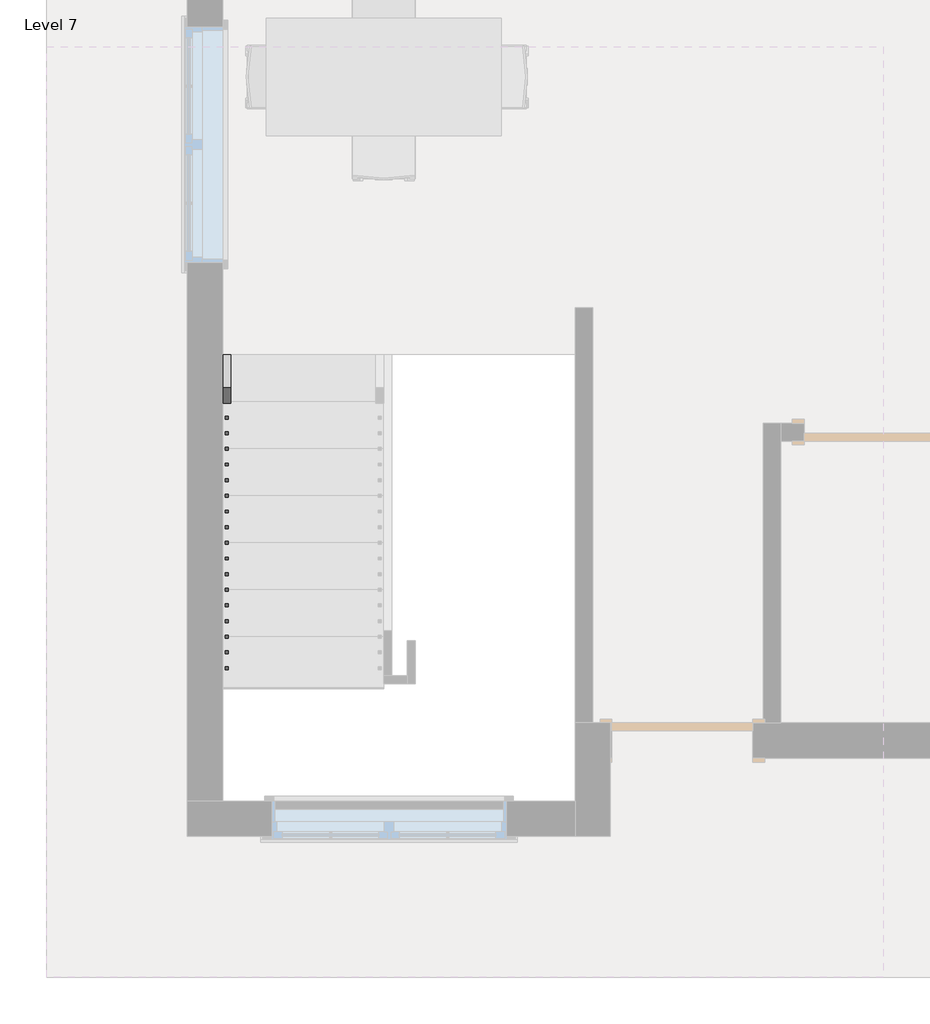
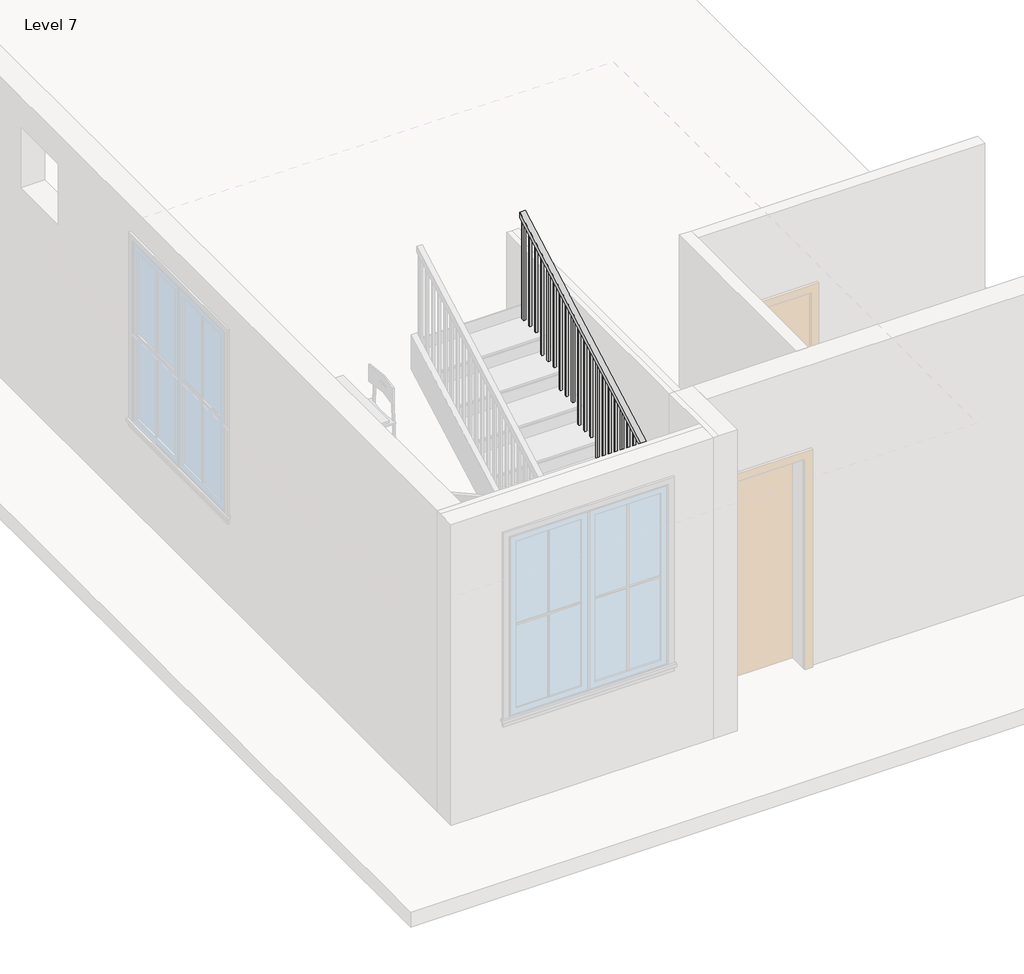
# One storey, part 2 of 3: 1 railing.
"""IFC4 building model written with IfcOpenShell, lengths in millimetres."""

from ifc_helpers import new_model, si_unit, frame, origin, place, context, project, spatial, polyline, outline, extrude, faceted_brep, element, save

model = new_model("IFC4")

# Units and contexts
model_context = context("Model", 3, world=origin())
ifc_project = project(units=[si_unit("LENGTHUNIT", "METRE", prefix="MILLI")], contexts=[model_context])

# Site, building, storey
site = spatial("IfcSite", under=ifc_project)
building = spatial("IfcBuilding", under=site)
storey = spatial("IfcBuildingStorey", under=building, Name="Level 7", Elevation=19050.0)

# Railing
placement = place(None, origin())
element("IfcRailing", 1, ObjectType="Handrail - Rectangular", at=placement, inside=storey, context=model_context, shape_type="SolidModel", body=[
    faceted_brep([(-4181.480864, -3571.6080018, 20133.7333333), (-4181.480864, -3571.6080018, 20075.620221), (-4232.280864, -3571.6080018, 20075.620221), (-4232.280864, -3571.6080018, 20133.7333333), (-4181.480864, -5705.2080018, 21319.0666667), (-4181.480864, -5718.371604, 21268.2666667), (-4232.280864, -5718.371604, 21268.2666667), (-4232.280864, -5705.2080018, 21319.0666667), (-4181.480864, -6416.4080018, 21319.0666667), (-4181.480864, -6416.4080018, 21268.2666667), (-4232.280864, -6467.2080018, 21268.2666667), (-4232.280864, -6467.2080018, 21319.0666667), (-1997.080864, -6416.4080018, 21319.0666667), (-1997.080864, -6416.4080018, 21268.2666667), (-1946.280864, -6467.2080018, 21268.2666667), (-1946.280864, -6467.2080018, 21319.0666667), (-1997.080864, -5705.2080018, 21319.0666667), (-1997.080864, -5692.0443995, 21268.2666667), (-1946.280864, -5692.0443995, 21268.2666667), (-1946.280864, -5705.2080018, 21319.0666667), (-1997.080864, -3571.6080018, 22504.4), (-1946.280864, -3571.6080018, 22504.4), (-1946.280864, -3571.6080018, 22446.2868876), (-1997.080864, -3571.6080018, 22446.2868876)], [[[0, 1, 2, 3]], [[1, 0, 4, 5]], [[2, 1, 5, 6]], [[3, 2, 6, 7]], [[0, 3, 7, 4]], [[5, 4, 8, 9]], [[6, 5, 9, 10]], [[7, 6, 10, 11]], [[4, 7, 11, 8]], [[9, 8, 12, 13]], [[10, 9, 13, 14]], [[11, 10, 14, 15]], [[8, 11, 15, 12]], [[13, 12, 16, 17]], [[14, 13, 17, 18]], [[15, 14, 18, 19]], [[12, 15, 19, 16]], [[20, 21, 22, 23]], [[17, 16, 20, 23]], [[18, 17, 23, 22]], [[19, 18, 22, 21]], [[16, 19, 21, 20]]]),
    extrude(outline(polyline([(-3606.5330018, 22426.8841099), (-3587.4830018, 22437.4674432), (-3587.4830018, 21420.6666667), (-3606.5330018, 21420.6666667), (-3606.5330018, 22426.8841099)])), frame((-1981.205864, 0.0, 0.0), z_axis=(1.0, 0.0, 0.0), x_axis=(0.0, 1.0, 0.0)), (0.0, 0.0, 1.0), 19.05),
    extrude(outline(polyline([(-3708.1330018, 22370.4396654), (-3689.0830018, 22381.0229988), (-3689.0830018, 21420.6666667), (-3708.1330018, 21420.6666667), (-3708.1330018, 22370.4396654)])), frame((-1981.205864, 0.0, 0.0), z_axis=(1.0, 0.0, 0.0), x_axis=(0.0, 1.0, 0.0)), (0.0, 0.0, 1.0), 19.05),
    extrude(outline(polyline([(-3809.7330018, 22313.995221), (-3790.6830018, 22324.5785543), (-3790.6830018, 21420.6666667), (-3809.7330018, 21420.6666667), (-3809.7330018, 22313.995221)])), frame((-1981.205864, 0.0, 0.0), z_axis=(1.0, 0.0, 0.0), x_axis=(0.0, 1.0, 0.0)), (0.0, 0.0, 1.0), 19.05),
    extrude(outline(polyline([(-3911.3330018, 22257.5507765), (-3892.2830018, 22268.1341099), (-3892.2830018, 21251.3333333), (-3911.3330018, 21251.3333333), (-3911.3330018, 22257.5507765)])), frame((-1981.205864, 0.0, 0.0), z_axis=(1.0, 0.0, 0.0), x_axis=(0.0, 1.0, 0.0)), (0.0, 0.0, 1.0), 19.05),
    extrude(outline(polyline([(-4012.9330018, 22201.1063321), (-3993.8830018, 22211.6896654), (-3993.8830018, 21251.3333333), (-4012.9330018, 21251.3333333), (-4012.9330018, 22201.1063321)])), frame((-1981.205864, 0.0, 0.0), z_axis=(1.0, 0.0, 0.0), x_axis=(0.0, 1.0, 0.0)), (0.0, 0.0, 1.0), 19.05),
    extrude(outline(polyline([(-4114.5330018, 22144.6618876), (-4095.4830018, 22155.245221), (-4095.4830018, 21251.3333333), (-4114.5330018, 21251.3333333), (-4114.5330018, 22144.6618876)])), frame((-1981.205864, 0.0, 0.0), z_axis=(1.0, 0.0, 0.0), x_axis=(0.0, 1.0, 0.0)), (0.0, 0.0, 1.0), 19.05),
    extrude(outline(polyline([(-4216.1330018, 22088.2174432), (-4197.0830018, 22098.8007765), (-4197.0830018, 21082.0), (-4216.1330018, 21082.0), (-4216.1330018, 22088.2174432)])), frame((-1981.205864, 0.0, 0.0), z_axis=(1.0, 0.0, 0.0), x_axis=(0.0, 1.0, 0.0)), (0.0, 0.0, 1.0), 19.05),
    extrude(outline(polyline([(-4317.7330018, 22031.7729988), (-4298.6830018, 22042.3563321), (-4298.6830018, 21082.0), (-4317.7330018, 21082.0), (-4317.7330018, 22031.7729988)])), frame((-1981.205864, 0.0, 0.0), z_axis=(1.0, 0.0, 0.0), x_axis=(0.0, 1.0, 0.0)), (0.0, 0.0, 1.0), 19.05),
    extrude(outline(polyline([(-4419.3330018, 21975.3285543), (-4400.2830018, 21985.9118876), (-4400.2830018, 21082.0), (-4419.3330018, 21082.0), (-4419.3330018, 21975.3285543)])), frame((-1981.205864, 0.0, 0.0), z_axis=(1.0, 0.0, 0.0), x_axis=(0.0, 1.0, 0.0)), (0.0, 0.0, 1.0), 19.05),
    extrude(outline(polyline([(-4520.9330018, 21918.8841099), (-4501.8830018, 21929.4674432), (-4501.8830018, 20912.6666667), (-4520.9330018, 20912.6666667), (-4520.9330018, 21918.8841099)])), frame((-1981.205864, 0.0, 0.0), z_axis=(1.0, 0.0, 0.0), x_axis=(0.0, 1.0, 0.0)), (0.0, 0.0, 1.0), 19.05),
    extrude(outline(polyline([(-4622.5330018, 21862.4396654), (-4603.4830018, 21873.0229988), (-4603.4830018, 20912.6666667), (-4622.5330018, 20912.6666667), (-4622.5330018, 21862.4396654)])), frame((-1981.205864, 0.0, 0.0), z_axis=(1.0, 0.0, 0.0), x_axis=(0.0, 1.0, 0.0)), (0.0, 0.0, 1.0), 19.05),
    extrude(outline(polyline([(-4724.1330018, 21805.995221), (-4705.0830018, 21816.5785543), (-4705.0830018, 20912.6666667), (-4724.1330018, 20912.6666667), (-4724.1330018, 21805.995221)])), frame((-1981.205864, 0.0, 0.0), z_axis=(1.0, 0.0, 0.0), x_axis=(0.0, 1.0, 0.0)), (0.0, 0.0, 1.0), 19.05),
    extrude(outline(polyline([(-4825.7330018, 21749.5507765), (-4806.6830018, 21760.1341099), (-4806.6830018, 20743.3333333), (-4825.7330018, 20743.3333333), (-4825.7330018, 21749.5507765)])), frame((-1981.205864, 0.0, 0.0), z_axis=(1.0, 0.0, 0.0), x_axis=(0.0, 1.0, 0.0)), (0.0, 0.0, 1.0), 19.05),
    extrude(outline(polyline([(-4927.3330018, 21693.1063321), (-4908.2830018, 21703.6896654), (-4908.2830018, 20743.3333333), (-4927.3330018, 20743.3333333), (-4927.3330018, 21693.1063321)])), frame((-1981.205864, 0.0, 0.0), z_axis=(1.0, 0.0, 0.0), x_axis=(0.0, 1.0, 0.0)), (0.0, 0.0, 1.0), 19.05),
    extrude(outline(polyline([(-5028.9330018, 21636.6618876), (-5009.8830018, 21647.245221), (-5009.8830018, 20743.3333333), (-5028.9330018, 20743.3333333), (-5028.9330018, 21636.6618876)])), frame((-1981.205864, 0.0, 0.0), z_axis=(1.0, 0.0, 0.0), x_axis=(0.0, 1.0, 0.0)), (0.0, 0.0, 1.0), 19.05),
    extrude(outline(polyline([(-5130.5330018, 21580.2174432), (-5111.4830018, 21590.8007765), (-5111.4830018, 20574.0), (-5130.5330018, 20574.0), (-5130.5330018, 21580.2174432)])), frame((-1981.205864, 0.0, 0.0), z_axis=(1.0, 0.0, 0.0), x_axis=(0.0, 1.0, 0.0)), (0.0, 0.0, 1.0), 19.05),
    extrude(outline(polyline([(-5232.1330018, 21523.7729988), (-5213.0830018, 21534.3563321), (-5213.0830018, 20574.0), (-5232.1330018, 20574.0), (-5232.1330018, 21523.7729988)])), frame((-1981.205864, 0.0, 0.0), z_axis=(1.0, 0.0, 0.0), x_axis=(0.0, 1.0, 0.0)), (0.0, 0.0, 1.0), 19.05),
    extrude(outline(polyline([(-5333.7330018, 21467.3285543), (-5314.6830018, 21477.9118876), (-5314.6830018, 20574.0), (-5333.7330018, 20574.0), (-5333.7330018, 21467.3285543)])), frame((-1981.205864, 0.0, 0.0), z_axis=(1.0, 0.0, 0.0), x_axis=(0.0, 1.0, 0.0)), (0.0, 0.0, 1.0), 19.05),
    extrude(outline(polyline([(-5435.3330018, 21410.8841099), (-5416.2830018, 21421.4674432), (-5416.2830018, 20404.6666667), (-5435.3330018, 20404.6666667), (-5435.3330018, 21410.8841099)])), frame((-1981.205864, 0.0, 0.0), z_axis=(1.0, 0.0, 0.0), x_axis=(0.0, 1.0, 0.0)), (0.0, 0.0, 1.0), 19.05),
    extrude(outline(polyline([(-5536.9330018, 21354.4396654), (-5517.8830018, 21365.0229988), (-5517.8830018, 20404.6666667), (-5536.9330018, 20404.6666667), (-5536.9330018, 21354.4396654)])), frame((-1981.205864, 0.0, 0.0), z_axis=(1.0, 0.0, 0.0), x_axis=(0.0, 1.0, 0.0)), (0.0, 0.0, 1.0), 19.05),
    extrude(outline(polyline([(-5638.5330018, 21297.995221), (-5619.4830018, 21308.5785543), (-5619.4830018, 20404.6666667), (-5638.5330018, 20404.6666667), (-5638.5330018, 21297.995221)])), frame((-1981.205864, 0.0, 0.0), z_axis=(1.0, 0.0, 0.0), x_axis=(0.0, 1.0, 0.0)), (0.0, 0.0, 1.0), 19.05),
    extrude(outline(polyline([(-1962.155864, -5740.1330018), (-1981.205864, -5740.1330018), (-1981.205864, -5721.0830018), (-1962.155864, -5721.0830018), (-1962.155864, -5740.1330018)])), frame((0.0, 0.0, 20404.6666667), z_axis=(0.0, 0.0, 1.0), x_axis=(1.0, 0.0, 0.0)), (0.0, 0.0, 1.0), 863.6),
    extrude(outline(polyline([(-1962.155864, -5841.7330018), (-1981.205864, -5841.7330018), (-1981.205864, -5822.6830018), (-1962.155864, -5822.6830018), (-1962.155864, -5841.7330018)])), frame((0.0, 0.0, 20404.6666667), z_axis=(0.0, 0.0, 1.0), x_axis=(1.0, 0.0, 0.0)), (0.0, 0.0, 1.0), 863.6),
    extrude(outline(polyline([(-1962.155864, -5943.3330018), (-1981.205864, -5943.3330018), (-1981.205864, -5924.2830018), (-1962.155864, -5924.2830018), (-1962.155864, -5943.3330018)])), frame((0.0, 0.0, 20404.6666667), z_axis=(0.0, 0.0, 1.0), x_axis=(1.0, 0.0, 0.0)), (0.0, 0.0, 1.0), 863.6),
    extrude(outline(polyline([(-1962.155864, -6044.9330018), (-1981.205864, -6044.9330018), (-1981.205864, -6025.8830018), (-1962.155864, -6025.8830018), (-1962.155864, -6044.9330018)])), frame((0.0, 0.0, 20404.6666667), z_axis=(0.0, 0.0, 1.0), x_axis=(1.0, 0.0, 0.0)), (0.0, 0.0, 1.0), 863.6),
    extrude(outline(polyline([(-1962.155864, -6146.5330018), (-1981.205864, -6146.5330018), (-1981.205864, -6127.4830018), (-1962.155864, -6127.4830018), (-1962.155864, -6146.5330018)])), frame((0.0, 0.0, 20404.6666667), z_axis=(0.0, 0.0, 1.0), x_axis=(1.0, 0.0, 0.0)), (0.0, 0.0, 1.0), 863.6),
    extrude(outline(polyline([(-1962.155864, -6248.1330018), (-1981.205864, -6248.1330018), (-1981.205864, -6229.0830018), (-1962.155864, -6229.0830018), (-1962.155864, -6248.1330018)])), frame((0.0, 0.0, 20404.6666667), z_axis=(0.0, 0.0, 1.0), x_axis=(1.0, 0.0, 0.0)), (0.0, 0.0, 1.0), 863.6),
    extrude(outline(polyline([(-1962.155864, -6349.7330018), (-1981.205864, -6349.7330018), (-1981.205864, -6330.6830018), (-1962.155864, -6330.6830018), (-1962.155864, -6349.7330018)])), frame((0.0, 0.0, 20404.6666667), z_axis=(0.0, 0.0, 1.0), x_axis=(1.0, 0.0, 0.0)), (0.0, 0.0, 1.0), 863.6),
    extrude(outline(polyline([(-2082.805864, -6451.3330018), (-2082.805864, -6432.2830018), (-2063.755864, -6432.2830018), (-2063.755864, -6451.3330018), (-2082.805864, -6451.3330018)])), frame((0.0, 0.0, 20404.6666667), z_axis=(0.0, 0.0, 1.0), x_axis=(1.0, 0.0, 0.0)), (0.0, 0.0, 1.0), 863.6),
    extrude(outline(polyline([(-2184.405864, -6451.3330018), (-2184.405864, -6432.2830018), (-2165.355864, -6432.2830018), (-2165.355864, -6451.3330018), (-2184.405864, -6451.3330018)])), frame((0.0, 0.0, 20404.6666667), z_axis=(0.0, 0.0, 1.0), x_axis=(1.0, 0.0, 0.0)), (0.0, 0.0, 1.0), 863.6),
    extrude(outline(polyline([(-2286.005864, -6451.3330018), (-2286.005864, -6432.2830018), (-2266.955864, -6432.2830018), (-2266.955864, -6451.3330018), (-2286.005864, -6451.3330018)])), frame((0.0, 0.0, 20404.6666667), z_axis=(0.0, 0.0, 1.0), x_axis=(1.0, 0.0, 0.0)), (0.0, 0.0, 1.0), 863.6),
    extrude(outline(polyline([(-2387.605864, -6451.3330018), (-2387.605864, -6432.2830018), (-2368.555864, -6432.2830018), (-2368.555864, -6451.3330018), (-2387.605864, -6451.3330018)])), frame((0.0, 0.0, 20404.6666667), z_axis=(0.0, 0.0, 1.0), x_axis=(1.0, 0.0, 0.0)), (0.0, 0.0, 1.0), 863.6),
    extrude(outline(polyline([(-2489.205864, -6451.3330018), (-2489.205864, -6432.2830018), (-2470.155864, -6432.2830018), (-2470.155864, -6451.3330018), (-2489.205864, -6451.3330018)])), frame((0.0, 0.0, 20404.6666667), z_axis=(0.0, 0.0, 1.0), x_axis=(1.0, 0.0, 0.0)), (0.0, 0.0, 1.0), 863.6),
    extrude(outline(polyline([(-2590.805864, -6451.3330018), (-2590.805864, -6432.2830018), (-2571.755864, -6432.2830018), (-2571.755864, -6451.3330018), (-2590.805864, -6451.3330018)])), frame((0.0, 0.0, 20404.6666667), z_axis=(0.0, 0.0, 1.0), x_axis=(1.0, 0.0, 0.0)), (0.0, 0.0, 1.0), 863.6),
    extrude(outline(polyline([(-2692.405864, -6451.3330018), (-2692.405864, -6432.2830018), (-2673.355864, -6432.2830018), (-2673.355864, -6451.3330018), (-2692.405864, -6451.3330018)])), frame((0.0, 0.0, 20404.6666667), z_axis=(0.0, 0.0, 1.0), x_axis=(1.0, 0.0, 0.0)), (0.0, 0.0, 1.0), 863.6),
    extrude(outline(polyline([(-2794.005864, -6451.3330018), (-2794.005864, -6432.2830018), (-2774.955864, -6432.2830018), (-2774.955864, -6451.3330018), (-2794.005864, -6451.3330018)])), frame((0.0, 0.0, 20404.6666667), z_axis=(0.0, 0.0, 1.0), x_axis=(1.0, 0.0, 0.0)), (0.0, 0.0, 1.0), 863.6),
    extrude(outline(polyline([(-2895.605864, -6451.3330018), (-2895.605864, -6432.2830018), (-2876.555864, -6432.2830018), (-2876.555864, -6451.3330018), (-2895.605864, -6451.3330018)])), frame((0.0, 0.0, 20404.6666667), z_axis=(0.0, 0.0, 1.0), x_axis=(1.0, 0.0, 0.0)), (0.0, 0.0, 1.0), 863.6),
    extrude(outline(polyline([(-2997.205864, -6451.3330018), (-2997.205864, -6432.2830018), (-2978.155864, -6432.2830018), (-2978.155864, -6451.3330018), (-2997.205864, -6451.3330018)])), frame((0.0, 0.0, 20404.6666667), z_axis=(0.0, 0.0, 1.0), x_axis=(1.0, 0.0, 0.0)), (0.0, 0.0, 1.0), 863.6),
    extrude(outline(polyline([(-3098.805864, -6451.3330018), (-3098.805864, -6432.2830018), (-3079.755864, -6432.2830018), (-3079.755864, -6451.3330018), (-3098.805864, -6451.3330018)])), frame((0.0, 0.0, 20404.6666667), z_axis=(0.0, 0.0, 1.0), x_axis=(1.0, 0.0, 0.0)), (0.0, 0.0, 1.0), 863.6),
    extrude(outline(polyline([(-3200.405864, -6451.3330018), (-3200.405864, -6432.2830018), (-3181.355864, -6432.2830018), (-3181.355864, -6451.3330018), (-3200.405864, -6451.3330018)])), frame((0.0, 0.0, 20404.6666667), z_axis=(0.0, 0.0, 1.0), x_axis=(1.0, 0.0, 0.0)), (0.0, 0.0, 1.0), 863.6),
    extrude(outline(polyline([(-3302.005864, -6451.3330018), (-3302.005864, -6432.2830018), (-3282.955864, -6432.2830018), (-3282.955864, -6451.3330018), (-3302.005864, -6451.3330018)])), frame((0.0, 0.0, 20404.6666667), z_axis=(0.0, 0.0, 1.0), x_axis=(1.0, 0.0, 0.0)), (0.0, 0.0, 1.0), 863.6),
    extrude(outline(polyline([(-3403.605864, -6451.3330018), (-3403.605864, -6432.2830018), (-3384.555864, -6432.2830018), (-3384.555864, -6451.3330018), (-3403.605864, -6451.3330018)])), frame((0.0, 0.0, 20404.6666667), z_axis=(0.0, 0.0, 1.0), x_axis=(1.0, 0.0, 0.0)), (0.0, 0.0, 1.0), 863.6),
    extrude(outline(polyline([(-3505.205864, -6451.3330018), (-3505.205864, -6432.2830018), (-3486.155864, -6432.2830018), (-3486.155864, -6451.3330018), (-3505.205864, -6451.3330018)])), frame((0.0, 0.0, 20404.6666667), z_axis=(0.0, 0.0, 1.0), x_axis=(1.0, 0.0, 0.0)), (0.0, 0.0, 1.0), 863.6),
    extrude(outline(polyline([(-3606.805864, -6451.3330018), (-3606.805864, -6432.2830018), (-3587.755864, -6432.2830018), (-3587.755864, -6451.3330018), (-3606.805864, -6451.3330018)])), frame((0.0, 0.0, 20404.6666667), z_axis=(0.0, 0.0, 1.0), x_axis=(1.0, 0.0, 0.0)), (0.0, 0.0, 1.0), 863.6),
    extrude(outline(polyline([(-3708.405864, -6451.3330018), (-3708.405864, -6432.2830018), (-3689.355864, -6432.2830018), (-3689.355864, -6451.3330018), (-3708.405864, -6451.3330018)])), frame((0.0, 0.0, 20404.6666667), z_axis=(0.0, 0.0, 1.0), x_axis=(1.0, 0.0, 0.0)), (0.0, 0.0, 1.0), 863.6),
    extrude(outline(polyline([(-3810.005864, -6451.3330018), (-3810.005864, -6432.2830018), (-3790.955864, -6432.2830018), (-3790.955864, -6451.3330018), (-3810.005864, -6451.3330018)])), frame((0.0, 0.0, 20404.6666667), z_axis=(0.0, 0.0, 1.0), x_axis=(1.0, 0.0, 0.0)), (0.0, 0.0, 1.0), 863.6),
    extrude(outline(polyline([(-3911.605864, -6451.3330018), (-3911.605864, -6432.2830018), (-3892.555864, -6432.2830018), (-3892.555864, -6451.3330018), (-3911.605864, -6451.3330018)])), frame((0.0, 0.0, 20404.6666667), z_axis=(0.0, 0.0, 1.0), x_axis=(1.0, 0.0, 0.0)), (0.0, 0.0, 1.0), 863.6),
    extrude(outline(polyline([(-4013.205864, -6451.3330018), (-4013.205864, -6432.2830018), (-3994.155864, -6432.2830018), (-3994.155864, -6451.3330018), (-4013.205864, -6451.3330018)])), frame((0.0, 0.0, 20404.6666667), z_axis=(0.0, 0.0, 1.0), x_axis=(1.0, 0.0, 0.0)), (0.0, 0.0, 1.0), 863.6),
    extrude(outline(polyline([(-4114.805864, -6451.3330018), (-4114.805864, -6432.2830018), (-4095.755864, -6432.2830018), (-4095.755864, -6451.3330018), (-4114.805864, -6451.3330018)])), frame((0.0, 0.0, 20404.6666667), z_axis=(0.0, 0.0, 1.0), x_axis=(1.0, 0.0, 0.0)), (0.0, 0.0, 1.0), 863.6),
    extrude(outline(polyline([(-4216.405864, -6406.8830018), (-4197.355864, -6406.8830018), (-4197.355864, -6425.9330018), (-4216.405864, -6425.9330018), (-4216.405864, -6406.8830018)])), frame((0.0, 0.0, 20404.6666667), z_axis=(0.0, 0.0, 1.0), x_axis=(1.0, 0.0, 0.0)), (0.0, 0.0, 1.0), 863.6),
    extrude(outline(polyline([(-4216.405864, -6305.2830018), (-4197.355864, -6305.2830018), (-4197.355864, -6324.3330018), (-4216.405864, -6324.3330018), (-4216.405864, -6305.2830018)])), frame((0.0, 0.0, 20404.6666667), z_axis=(0.0, 0.0, 1.0), x_axis=(1.0, 0.0, 0.0)), (0.0, 0.0, 1.0), 863.6),
    extrude(outline(polyline([(-4216.405864, -6203.6830018), (-4197.355864, -6203.6830018), (-4197.355864, -6222.7330018), (-4216.405864, -6222.7330018), (-4216.405864, -6203.6830018)])), frame((0.0, 0.0, 20404.6666667), z_axis=(0.0, 0.0, 1.0), x_axis=(1.0, 0.0, 0.0)), (0.0, 0.0, 1.0), 863.6),
    extrude(outline(polyline([(-4216.405864, -6102.0830018), (-4197.355864, -6102.0830018), (-4197.355864, -6121.1330018), (-4216.405864, -6121.1330018), (-4216.405864, -6102.0830018)])), frame((0.0, 0.0, 20404.6666667), z_axis=(0.0, 0.0, 1.0), x_axis=(1.0, 0.0, 0.0)), (0.0, 0.0, 1.0), 863.6),
    extrude(outline(polyline([(-4216.405864, -6000.4830018), (-4197.355864, -6000.4830018), (-4197.355864, -6019.5330018), (-4216.405864, -6019.5330018), (-4216.405864, -6000.4830018)])), frame((0.0, 0.0, 20404.6666667), z_axis=(0.0, 0.0, 1.0), x_axis=(1.0, 0.0, 0.0)), (0.0, 0.0, 1.0), 863.6),
    extrude(outline(polyline([(-4216.405864, -5898.8830018), (-4197.355864, -5898.8830018), (-4197.355864, -5917.9330018), (-4216.405864, -5917.9330018), (-4216.405864, -5898.8830018)])), frame((0.0, 0.0, 20404.6666667), z_axis=(0.0, 0.0, 1.0), x_axis=(1.0, 0.0, 0.0)), (0.0, 0.0, 1.0), 863.6),
    extrude(outline(polyline([(-4216.405864, -5797.2830018), (-4197.355864, -5797.2830018), (-4197.355864, -5816.3330018), (-4216.405864, -5816.3330018), (-4216.405864, -5797.2830018)])), frame((0.0, 0.0, 20404.6666667), z_axis=(0.0, 0.0, 1.0), x_axis=(1.0, 0.0, 0.0)), (0.0, 0.0, 1.0), 863.6),
    extrude(outline(polyline([(-5714.7330018, 21266.245221), (-5695.6830018, 21255.6618876), (-5695.6830018, 20404.6666667), (-5714.7330018, 20404.6666667), (-5714.7330018, 21266.245221)])), frame((-4216.405864, 0.0, 0.0), z_axis=(1.0, 0.0, 0.0), x_axis=(0.0, 1.0, 0.0)), (0.0, 0.0, 1.0), 19.05),
    extrude(outline(polyline([(-5613.1330018, 21209.8007765), (-5594.0830018, 21199.2174432), (-5594.0830018, 20235.3333333), (-5613.1330018, 20235.3333333), (-5613.1330018, 21209.8007765)])), frame((-4216.405864, 0.0, 0.0), z_axis=(1.0, 0.0, 0.0), x_axis=(0.0, 1.0, 0.0)), (0.0, 0.0, 1.0), 19.05),
    extrude(outline(polyline([(-5511.5330018, 21153.3563321), (-5492.4830018, 21142.7729988), (-5492.4830018, 20235.3333333), (-5511.5330018, 20235.3333333), (-5511.5330018, 21153.3563321)])), frame((-4216.405864, 0.0, 0.0), z_axis=(1.0, 0.0, 0.0), x_axis=(0.0, 1.0, 0.0)), (0.0, 0.0, 1.0), 19.05),
    extrude(outline(polyline([(-5409.9330018, 21096.9118876), (-5390.8830018, 21086.3285543), (-5390.8830018, 20235.3333333), (-5409.9330018, 20235.3333333), (-5409.9330018, 21096.9118876)])), frame((-4216.405864, 0.0, 0.0), z_axis=(1.0, 0.0, 0.0), x_axis=(0.0, 1.0, 0.0)), (0.0, 0.0, 1.0), 19.05),
    extrude(outline(polyline([(-5308.3330018, 21040.4674432), (-5289.2830018, 21029.8841099), (-5289.2830018, 20066.0), (-5308.3330018, 20066.0), (-5308.3330018, 21040.4674432)])), frame((-4216.405864, 0.0, 0.0), z_axis=(1.0, 0.0, 0.0), x_axis=(0.0, 1.0, 0.0)), (0.0, 0.0, 1.0), 19.05),
    extrude(outline(polyline([(-5206.7330018, 20984.0229988), (-5187.6830018, 20973.4396654), (-5187.6830018, 20066.0), (-5206.7330018, 20066.0), (-5206.7330018, 20984.0229988)])), frame((-4216.405864, 0.0, 0.0), z_axis=(1.0, 0.0, 0.0), x_axis=(0.0, 1.0, 0.0)), (0.0, 0.0, 1.0), 19.05),
    extrude(outline(polyline([(-5105.1330018, 20927.5785543), (-5086.0830018, 20916.995221), (-5086.0830018, 20066.0), (-5105.1330018, 20066.0), (-5105.1330018, 20927.5785543)])), frame((-4216.405864, 0.0, 0.0), z_axis=(1.0, 0.0, 0.0), x_axis=(0.0, 1.0, 0.0)), (0.0, 0.0, 1.0), 19.05),
    extrude(outline(polyline([(-5003.5330018, 20871.1341099), (-4984.4830018, 20860.5507765), (-4984.4830018, 19896.6666667), (-5003.5330018, 19896.6666667), (-5003.5330018, 20871.1341099)])), frame((-4216.405864, 0.0, 0.0), z_axis=(1.0, 0.0, 0.0), x_axis=(0.0, 1.0, 0.0)), (0.0, 0.0, 1.0), 19.05),
    extrude(outline(polyline([(-4901.9330018, 20814.6896654), (-4882.8830018, 20804.1063321), (-4882.8830018, 19896.6666667), (-4901.9330018, 19896.6666667), (-4901.9330018, 20814.6896654)])), frame((-4216.405864, 0.0, 0.0), z_axis=(1.0, 0.0, 0.0), x_axis=(0.0, 1.0, 0.0)), (0.0, 0.0, 1.0), 19.05),
    extrude(outline(polyline([(-4800.3330018, 20758.245221), (-4781.2830018, 20747.6618876), (-4781.2830018, 19896.6666667), (-4800.3330018, 19896.6666667), (-4800.3330018, 20758.245221)])), frame((-4216.405864, 0.0, 0.0), z_axis=(1.0, 0.0, 0.0), x_axis=(0.0, 1.0, 0.0)), (0.0, 0.0, 1.0), 19.05),
    extrude(outline(polyline([(-4698.7330018, 20701.8007765), (-4679.6830018, 20691.2174432), (-4679.6830018, 19727.3333333), (-4698.7330018, 19727.3333333), (-4698.7330018, 20701.8007765)])), frame((-4216.405864, 0.0, 0.0), z_axis=(1.0, 0.0, 0.0), x_axis=(0.0, 1.0, 0.0)), (0.0, 0.0, 1.0), 19.05),
    extrude(outline(polyline([(-4597.1330018, 20645.3563321), (-4578.0830018, 20634.7729988), (-4578.0830018, 19727.3333333), (-4597.1330018, 19727.3333333), (-4597.1330018, 20645.3563321)])), frame((-4216.405864, 0.0, 0.0), z_axis=(1.0, 0.0, 0.0), x_axis=(0.0, 1.0, 0.0)), (0.0, 0.0, 1.0), 19.05),
    extrude(outline(polyline([(-4495.5330018, 20588.9118876), (-4476.4830018, 20578.3285543), (-4476.4830018, 19727.3333333), (-4495.5330018, 19727.3333333), (-4495.5330018, 20588.9118876)])), frame((-4216.405864, 0.0, 0.0), z_axis=(1.0, 0.0, 0.0), x_axis=(0.0, 1.0, 0.0)), (0.0, 0.0, 1.0), 19.05),
    extrude(outline(polyline([(-4393.9330018, 20532.4674432), (-4374.8830018, 20521.8841099), (-4374.8830018, 19558.0), (-4393.9330018, 19558.0), (-4393.9330018, 20532.4674432)])), frame((-4216.405864, 0.0, 0.0), z_axis=(1.0, 0.0, 0.0), x_axis=(0.0, 1.0, 0.0)), (0.0, 0.0, 1.0), 19.05),
    extrude(outline(polyline([(-4292.3330018, 20476.0229988), (-4273.2830018, 20465.4396654), (-4273.2830018, 19558.0), (-4292.3330018, 19558.0), (-4292.3330018, 20476.0229988)])), frame((-4216.405864, 0.0, 0.0), z_axis=(1.0, 0.0, 0.0), x_axis=(0.0, 1.0, 0.0)), (0.0, 0.0, 1.0), 19.05),
    extrude(outline(polyline([(-4190.7330018, 20419.5785543), (-4171.6830018, 20408.995221), (-4171.6830018, 19558.0), (-4190.7330018, 19558.0), (-4190.7330018, 20419.5785543)])), frame((-4216.405864, 0.0, 0.0), z_axis=(1.0, 0.0, 0.0), x_axis=(0.0, 1.0, 0.0)), (0.0, 0.0, 1.0), 19.05),
    extrude(outline(polyline([(-4089.1330018, 20363.1341099), (-4070.0830018, 20352.5507765), (-4070.0830018, 19388.6666667), (-4089.1330018, 19388.6666667), (-4089.1330018, 20363.1341099)])), frame((-4216.405864, 0.0, 0.0), z_axis=(1.0, 0.0, 0.0), x_axis=(0.0, 1.0, 0.0)), (0.0, 0.0, 1.0), 19.05),
    extrude(outline(polyline([(-3987.5330018, 20306.6896654), (-3968.4830018, 20296.1063321), (-3968.4830018, 19388.6666667), (-3987.5330018, 19388.6666667), (-3987.5330018, 20306.6896654)])), frame((-4216.405864, 0.0, 0.0), z_axis=(1.0, 0.0, 0.0), x_axis=(0.0, 1.0, 0.0)), (0.0, 0.0, 1.0), 19.05),
    extrude(outline(polyline([(-3885.9330018, 20250.245221), (-3866.8830018, 20239.6618876), (-3866.8830018, 19388.6666667), (-3885.9330018, 19388.6666667), (-3885.9330018, 20250.245221)])), frame((-4216.405864, 0.0, 0.0), z_axis=(1.0, 0.0, 0.0), x_axis=(0.0, 1.0, 0.0)), (0.0, 0.0, 1.0), 19.05),
    extrude(outline(polyline([(-3784.3330018, 20193.8007765), (-3765.2830018, 20183.2174432), (-3765.2830018, 19219.3333333), (-3784.3330018, 19219.3333333), (-3784.3330018, 20193.8007765)])), frame((-4216.405864, 0.0, 0.0), z_axis=(1.0, 0.0, 0.0), x_axis=(0.0, 1.0, 0.0)), (0.0, 0.0, 1.0), 19.05),
    extrude(outline(polyline([(-3682.7330018, 20137.3563321), (-3663.6830018, 20126.7729988), (-3663.6830018, 19219.3333333), (-3682.7330018, 19219.3333333), (-3682.7330018, 20137.3563321)])), frame((-4216.405864, 0.0, 0.0), z_axis=(1.0, 0.0, 0.0), x_axis=(0.0, 1.0, 0.0)), (0.0, 0.0, 1.0), 19.05),
    extrude(outline(polyline([(-1981.205864, -6451.3330018), (-1981.205864, -6432.2830018), (-1962.155864, -6432.2830018), (-1962.155864, -6451.3330018), (-1981.205864, -6451.3330018)])), frame((0.0, 0.0, 20404.6666667), z_axis=(0.0, 0.0, 1.0), x_axis=(1.0, 0.0, 0.0)), (0.0, 0.0, 1.0), 863.6),
    extrude(outline(polyline([(-4216.405864, -6432.2830018), (-4197.355864, -6432.2830018), (-4197.355864, -6451.3330018), (-4216.405864, -6451.3330018), (-4216.405864, -6432.2830018)])), frame((0.0, 0.0, 20404.6666667), z_axis=(0.0, 0.0, 1.0), x_axis=(1.0, 0.0, 0.0)), (0.0, 0.0, 1.0), 863.6),
    extrude(outline(polyline([(-3590.6580018, 22435.7035543), (-3571.6080018, 22446.2868876), (-3571.6080018, 21420.6666667), (-3590.6580018, 21420.6666667), (-3590.6580018, 22435.7035543)])), frame((-1981.205864, 0.0, 0.0), z_axis=(1.0, 0.0, 0.0), x_axis=(0.0, 1.0, 0.0)), (0.0, 0.0, 1.0), 19.05),
    extrude(outline(polyline([(-3590.6580018, 20086.2035543), (-3571.6080018, 20075.620221), (-3571.6080018, 19219.3333333), (-3590.6580018, 19219.3333333), (-3590.6580018, 20086.2035543)])), frame((-4216.405864, 0.0, 0.0), z_axis=(1.0, 0.0, 0.0), x_axis=(0.0, 1.0, 0.0)), (0.0, 0.0, 1.0), 19.05),
])

save(model, "model.ifc")

# Revit data of these elements
# Type "Handrail - Rectangular"
#   Assembly Code = "C2010400"
#   built-in parameter 1008612 = 0.0416667 (stored number, unit not read)
#   built-in parameter 1008611 = 0.0416667 (stored number, unit not read)
#   built-in parameter 1008609 = 0.333333 (stored number, unit not read)
#   built-in parameter 1008604 = 0.166667 (stored number, unit not read)
#   built-in parameter 1008603 = 0.166667 (stored number, unit not read)
#   Railing Height = 3' - 0"
#   built-in parameter 1008630 = 2
#   built-in parameter 1008610 = 2
#   built-in parameter 1008618 = Baluster - Square : 3/4"
# Element 1 (IfcRailing, "Handrail - Rectangular")
#   Phase Created = New Construction
